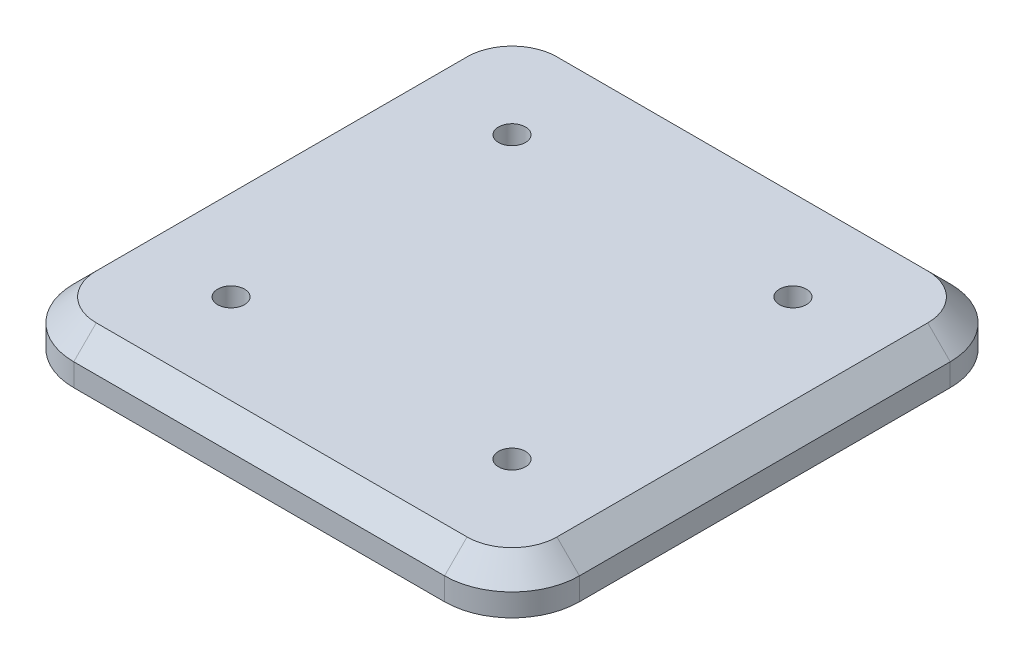
SolidWorks part; units mm, degrees
material "Plain Carbon Steel"
ref_plane "Front Plane" through (0, 0, 0) normal (0, 0, 1) x (1, 0, 0)
ref_plane "Top Plane" through (0, 0, 0) normal (0, 1, 0) x (1, 0, 0)
ref_plane "Right Plane" through (0, 0, 0) normal (1, 0, 0) x (0, 0, -1)
sketch "Base Plate Sketch 225x225" plane through (0, 0, 0) normal (0, 1, 0) x (1, 0, 0)
  line L1 (-112.5, -112.5) -> (112.5, -112.5)
  line L2 (-112.5, -112.5) -> (-112.5, 112.5)
  line L3 (-112.5, 112.5) -> (112.5, 112.5)
  line L4 (112.5, -112.5) -> (112.5, 112.5)
  line L5 (-112.5, -112.5) -> (112.5, 112.5) construction
  line L6 (-112.5, 112.5) -> (112.5, -112.5) construction
  point P0 (0, 0)
  dimension "D1" = 225
  dimension "D2" = 225
extrude "Base Plate 225x225x20" add sketch "Base Plate Sketch 225x225" along normal blind 20
fillet "Corner Fillets R30" radius 30 4 edges at (-112.5, 10, -112.5) (112.5, 10, -112.5) (112.5, 10, 112.5) (-112.5, 10, 112.5)
chamfer "Edge Chamfer 10x45" distance 10 angle 45 8 edges at (-112.5, 20, 0) (-103.7132, 20, 103.7132) (-103.7132, 20, -103.7132) (0, 20, 112.5) (0, 20, -112.5) (103.7132, 20, 103.7132) (103.7132, 20, -103.7132) (112.5, 20, 0)
sketch "Dowel Layout 125 Sketch" plane through (0, 20, 0) normal (0, 1, 0) x (1, 0, 0)
  line L1 (62.5, 62.5) -> (-62.5, 62.5)
  line L2 (62.5, 62.5) -> (62.5, -62.5)
  line L3 (62.5, -62.5) -> (-62.5, -62.5)
  line L4 (-62.5, 62.5) -> (-62.5, -62.5)
  line L5 (62.5, 62.5) -> (-62.5, -62.5) construction
  line L6 (62.5, -62.5) -> (-62.5, 62.5) construction
  point P0 (0, 0)
  dimension "D1" = 125
  dimension "D2" = 125
hole_wizard "Dowel Holes Ø12 on 125 Layout" positions "3DSketch1" profile "Sketch3" hole size "Ø12.0" standard "ANSI Metric"
sketch3d "3DSketch1"
  point P0 (62.5, 20, 62.5)
  point P3 (-62.5, 20, 62.5)
  point P6 (-62.5, 20, -62.5)
  point P9 (62.5, 20, -62.5)
sketch "Sketch3" plane through (62.5, 20, 62.5) normal (1, 0, 0) x (0, 0, 1)
  line L0 (0, 0) -> (0, 13.6052)
  line L1 (0, 13.6052) -> (6, 10)
  line L2 (6, 10) -> (6, 0)
  line L5 (6, 0) -> (0, 0)
  line L10 (0, 13.6052) -> (-6, 10) construction
  line L11 (0, -6.35) -> (0, 107.95) construction
  dimension "Hole Dia." = 12
  dimension "Hole Depth" = 10
  dimension "Drill Angle" = 118
sketch "Dowel Layout 175 Sketch" plane through (0, 0, 0) normal (0, -1, 0) x (1, 0, 0)
  line L1 (-87.5, -87.5) -> (87.5, -87.5)
  line L2 (-87.5, -87.5) -> (-87.5, 87.5)
  line L3 (-87.5, 87.5) -> (87.5, 87.5)
  line L4 (87.5, -87.5) -> (87.5, 87.5)
  line L5 (-87.5, -87.5) -> (87.5, 87.5) construction
  line L6 (-87.5, 87.5) -> (87.5, -87.5) construction
  point P0 (0, 0)
  dimension "D1" = 175
  dimension "D2" = 175
hole_wizard "Dowel Holes Ø12 on 175 Layout" positions "3DSketch2" profile "Sketch5" hole size "Ø12.0" standard "ANSI Metric"
sketch3d "3DSketch2"
  point P0 (-87.5, 0, 87.5)
  point P3 (87.5, 0, 87.5)
  point P6 (87.5, 0, -87.5)
  point P9 (-87.5, 0, -87.5)
sketch "Sketch5" plane through (-87.5, 0, 87.5) normal (1, 0, 0) x (0, 0, -1)
  line L0 (0, 0) -> (0, 13.6052)
  line L1 (0, 13.6052) -> (6, 10)
  line L2 (6, 10) -> (6, 0)
  line L5 (6, 0) -> (0, 0)
  line L10 (0, 13.6052) -> (-6, 10) construction
  line L11 (0, -6.35) -> (0, 107.95) construction
  dimension "Hole Dia." = 12
  dimension "Hole Depth" = 10
  dimension "Drill Angle" = 118
